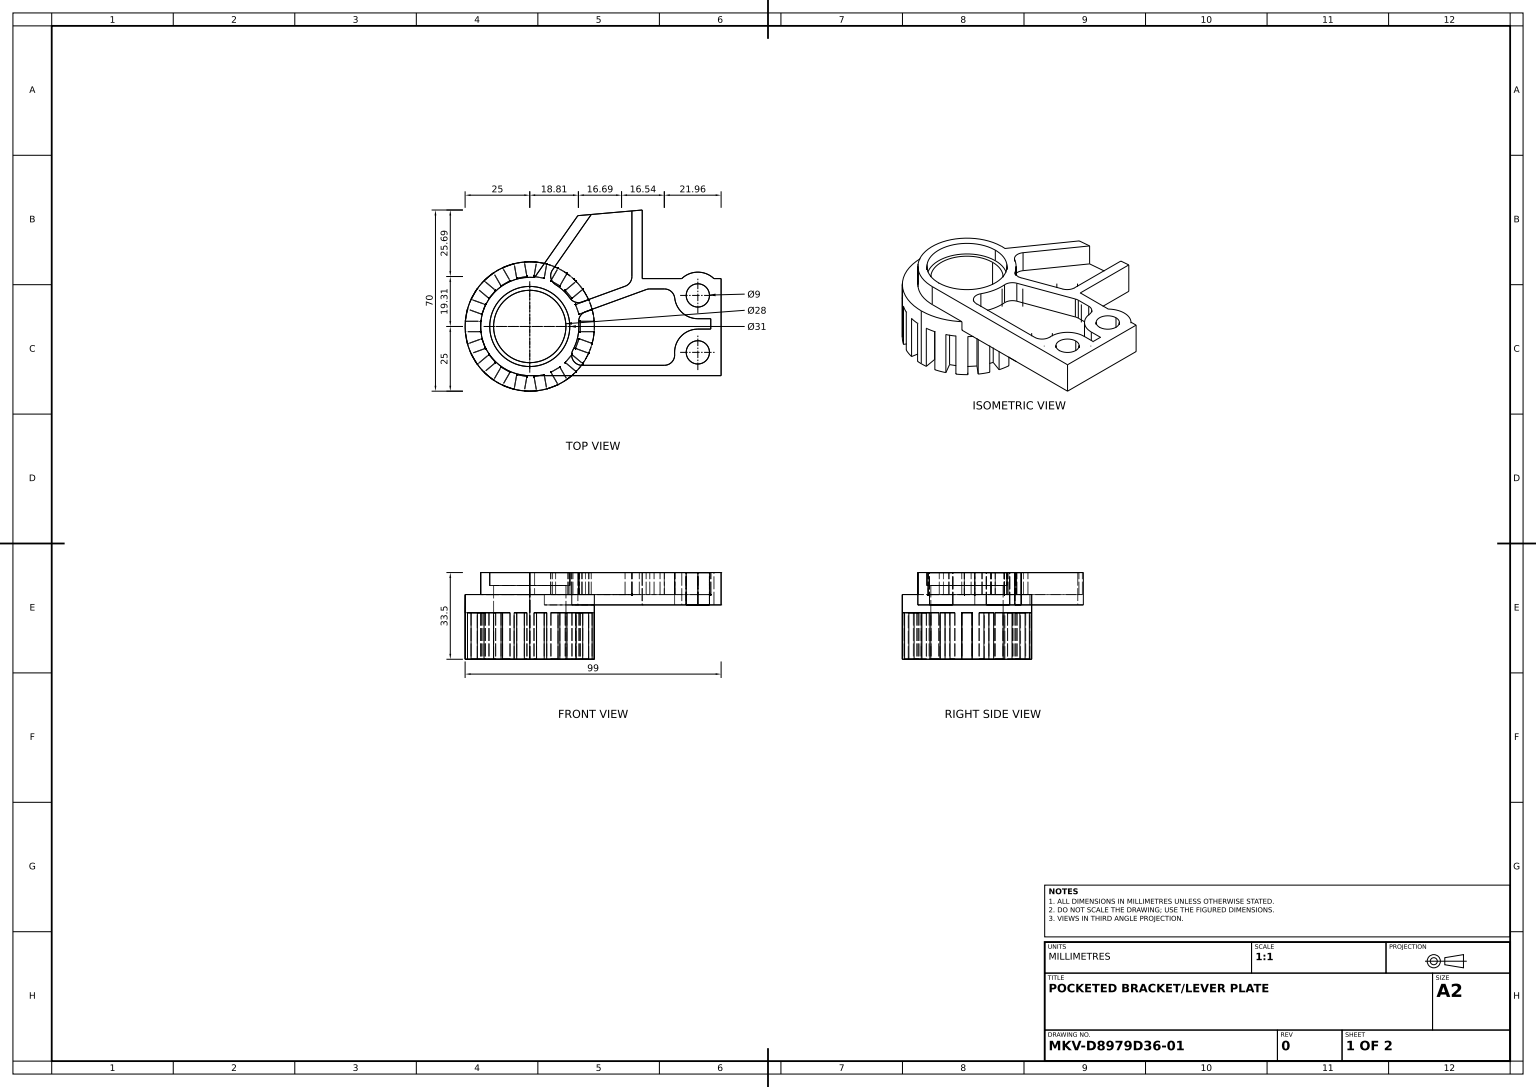
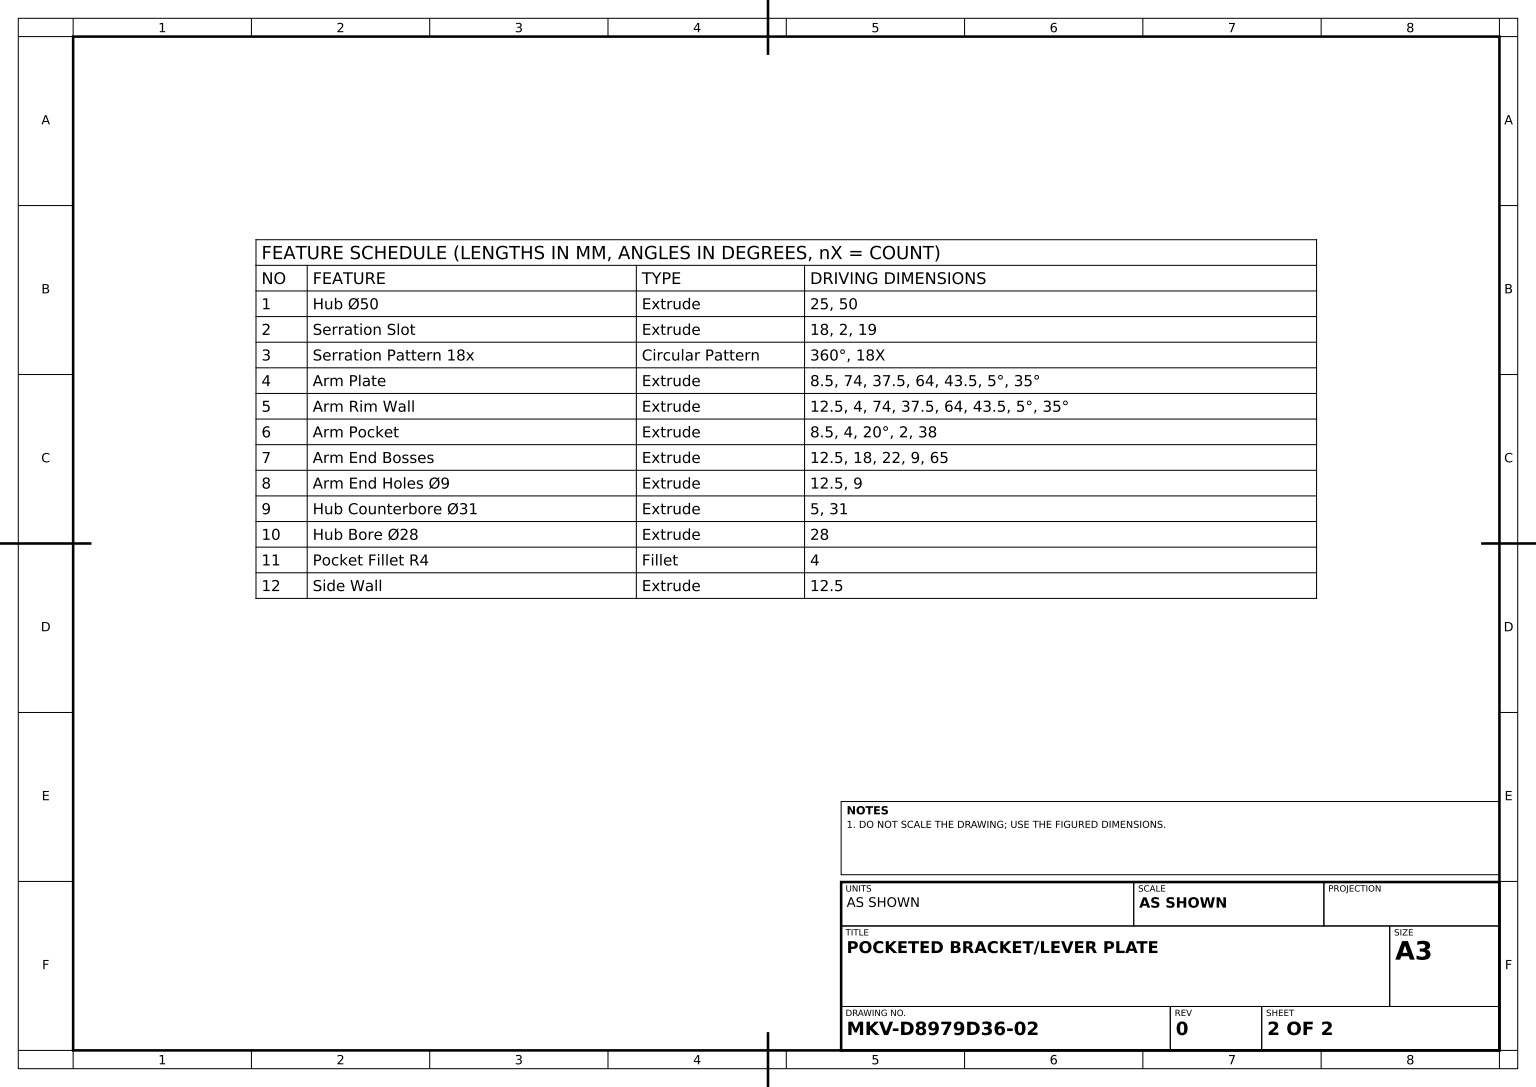
from build123d import *

# Parameters (mm, degrees)
HUB_PROFILE_50_R             = 25
HUB_50_DEPTH                 = 25
SERRATION_START              = -18
SERRATION_SLOT_DEPTH         = 18
SERRATION_PATTERN_18X_COUNT  = 18
ARM_OUTLINE_PROFILE_R        = 19
ARM_PLATE_DEPTH              = 8.5
ARM_START                    = -4
ARM_RIM_WALL_DEPTH           = 12.5
ARM_START_2                  = -8.5
ARM_POCKET_DEPTH             = 8.5
ARM_END_BOSS_PROFILE_R       = 9
ARM_END_BOSSES_DEPTH         = 12.5
ARM_END_HOLE_PROFILE_9_R     = 4.5
ARM_END_HOLES_9_DEPTH        = 12.5
HUB_COUNTERBORE_PROFILE_31_R = 15.5
HUB_COUNTERBORE_31_DEPTH     = 5
HUB_BORE_PROFILE_28_R        = 14
HUB_BORE_28_DEPTH            = 92.177025615
POCKET_FILLET_R4_R           = 4
SIDE_WALL_DEPTH              = 12.5


with BuildPart() as part:
    # Hub Profile _50 → Hub _50 (new body)
    with BuildSketch(Plane(origin=(0, 0, 0), x_dir=(1, 0, 0), z_dir=(0, 1, 0))):
        with Locations(Location((0, 0, 0), (0, 0, 270))):
            Circle(HUB_PROFILE_50_R)
    extrude(amount=-HUB_50_DEPTH)

    # Serration Slot Profile → Serration Slot (cut)
    with BuildSketch(Plane.XZ.offset(25).offset(SERRATION_START)):
        with BuildLine():
            Line((-19, 2), (-24.919871589, 2))
            ThreePointArc((-24.919871589, 2), (-25, 0), (-24.919871589, -2))
            Line((-24.919871589, -2), (-19, -2))
            Line((-19, -2), (-19, 2))
        make_face()
    serration_slot = extrude(amount=SERRATION_SLOT_DEPTH, mode=Mode.SUBTRACT)

    # Serration Pattern 18x: Serration Slot ×18 about axis
    serration_pattern_18x_axis = Axis((0.270845918, 0, 0), (0, 1, 0))
    for i in range(1, SERRATION_PATTERN_18X_COUNT):
        add(serration_slot.rotate(serration_pattern_18x_axis, i * 360 / SERRATION_PATTERN_18X_COUNT), mode=Mode.SUBTRACT)

    # Arm Outline Profile → Arm Plate (add)
    with BuildSketch(Plane(origin=(0, 0, 0), x_dir=(1, 0, 0), z_dir=(0, 1, 0))):
        with Locations(Location((0, 0, 0), (0, 0, 270))):
            Circle(ARM_OUTLINE_PROFILE_R)
    extrude(amount=ARM_PLATE_DEPTH)

    # Sketch3_5 → Arm Rim Wall (add)
    with BuildSketch(Plane(origin=(0, 0, 0), x_dir=(1, 0, 0), z_dir=(0, 1, 0)).offset(ARM_START)):
        with BuildLine():
            ThreePointArc((19, 0), (13.435028843, -13.435028843), (0, -19))
            Line((0, -19), (74, -19))
            Line((74, -19), (74, 18.5))
            Line((74, 18.5), (43.5, 18.5))
            Line((43.5, 18.5), (43.5, 45))
            Line((43.5, 45), (18.595132548, 42.821106431))
            Line((18.595132548, 42.821106431), (1.852058249, 18.909518245))
            ThreePointArc((1.852058249, 18.909518245), (14.074606686, 12.763441802), (19, 0))
        make_face()
    extrude(amount=ARM_RIM_WALL_DEPTH)

    # Arm Pocket Profile → Arm Pocket (cut)
    with BuildSketch(Plane(origin=(0, 8.5, 0), x_dir=(1, 0, 0), z_dir=(0, 1, 0)).offset(ARM_START_2)):
        with BuildLine():
            ThreePointArc((45.023258732, 14.258770483), (45.696746595, 14.439231012), (46.391339305, 14.5))
            Line((46.391339305, 14.5), (70, 14.5))
            Line((70, 14.5), (70, -15))
            Line((70, -15), (20.199009877, -15))
            ThreePointArc((20.199009877, -15), (16.760102062, -13.043015674), (16.686138594, -9.086956522))
            ThreePointArc((16.686138594, -9.086956522), (18.595302437, -3.900606013), (18.931172951, 1.61576319))
            ThreePointArc((18.931172951, 1.61576319), (19.545401033, 4.1087029), (21.548602473, 5.714694345))
            Line((21.548602473, 5.714694345), (45.023258732, 14.258770483))
        make_face()
        with BuildLine():
            Line((23.79689183, 43.276201399), (21.871740725, 40.526800686))
            Line((21.871740725, 40.526800686), (8.805008905, 21.865573683))
            ThreePointArc((8.805008905, 21.865573683), (8.164106806, 18.763113723), (9.980466285, 16.167569166))
            ThreePointArc((9.980466285, 16.167569166), (13.026439067, 13.831553971), (15.5407124, 10.930976996))
            ThreePointArc((15.5407124, 10.930976996), (17.613669166, 9.416092585), (20.1805219, 9.473464828))
            Line((20.1805219, 9.473464828), (36.868080573, 15.547239468))
            ThreePointArc((36.868080573, 15.547239468), (38.776608177, 17.011704206), (39.5, 19.306009951))
            Line((39.5, 19.306009951), (39.5, 44.650045346))
            Line((39.5, 44.650045346), (23.79689183, 43.276201399))
        make_face()
    extrude(amount=ARM_POCKET_DEPTH, mode=Mode.SUBTRACT)

    # Arm End Boss Profile → Arm End Bosses (add)
    with BuildSketch(Plane(origin=(0, 8.5, 0), x_dir=(1, 0, 0), z_dir=(0, 1, 0))):
        with Locations((65, 12)):
            Circle(ARM_END_BOSS_PROFILE_R)
        with Locations((65, -10)):
            Circle(ARM_END_BOSS_PROFILE_R)
    extrude(amount=-ARM_END_BOSSES_DEPTH)

    # Arm End Hole Profile _9 → Arm End Holes _9 (cut)
    with BuildSketch(Plane(origin=(0, 8.5, 0), x_dir=(1, 0, 0), z_dir=(0, 1, 0))):
        with Locations(Location((65, 12, 0), (0, 0, 270))):
            Circle(ARM_END_HOLE_PROFILE_9_R)
        with Locations(Location((65, -10, 0), (0, 0, 270))):
            Circle(ARM_END_HOLE_PROFILE_9_R)
    extrude(amount=-ARM_END_HOLES_9_DEPTH, mode=Mode.SUBTRACT)

    # Hub Counterbore Profile _31 → Hub Counterbore _31 (cut)
    with BuildSketch(Plane(origin=(0, 8.5, 0), x_dir=(1, 0, 0), z_dir=(0, 1, 0))):
        with Locations(Location((0, 0, 0), (0, 0, 270))):
            Circle(HUB_COUNTERBORE_PROFILE_31_R)
    extrude(amount=-HUB_COUNTERBORE_31_DEPTH, mode=Mode.SUBTRACT)

    # Hub Bore Profile _28 → Hub Bore _28 (cut, through all)
    with BuildSketch(Plane(origin=(0, 3.5, 0), x_dir=(1, 0, 0), z_dir=(0, 1, 0))):
        with Locations(Location((0, 0, 0), (0, 0, 270))):
            Circle(HUB_BORE_PROFILE_28_R)
    extrude(amount=-HUB_BORE_28_DEPTH, mode=Mode.SUBTRACT)

    # Pocket Fillet R4
    pocket_fillet_r4_edges = [part.edges().sort_by_distance(p)[0] for p in [
        (56.354191767, 4.25, -14.5),
        (57.516685226, 4.25, 15),
    ]]
    fillet(pocket_fillet_r4_edges, radius=POCKET_FILLET_R4_R)

    # Side Wall Profile → Side Wall (add)
    with BuildSketch(Plane(origin=(0, 8.5, 0), x_dir=(1, 0, 0), z_dir=(0, 1, 0))):
        with BuildLine():
            Line((65, 3), (70, 3))
            Line((70, 3), (70, 4.516685226))
            ThreePointArc((70, 4.516685226), (67.61248608, 3.38751392), (65, 3))
        make_face()
        with BuildLine():
            Line((65, -1), (70, -1))
            Line((70, -1), (70, -2.516685226))
            ThreePointArc((70, -2.516685226), (67.61248608, -1.38751392), (65, -1))
        make_face()
    extrude(amount=-SIDE_WALL_DEPTH)


solid = part.part
